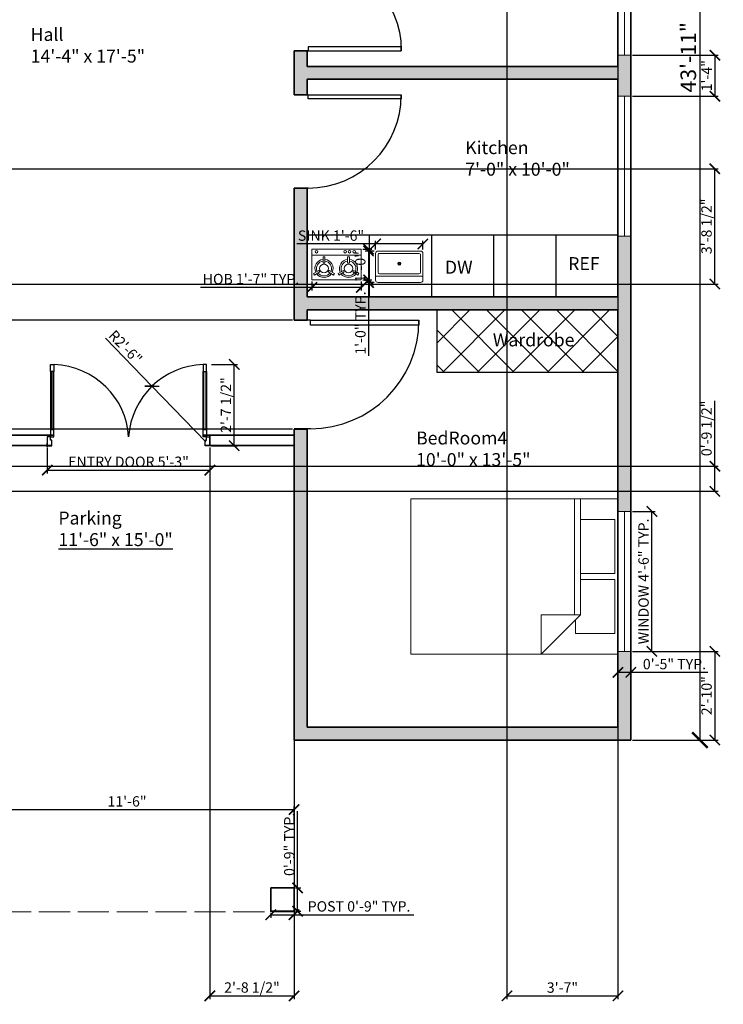
# Model space of a CAD drawing. Units: inches. Extents: x -43 to 8979, y -615 to 8149.
# Tile 2 of 5: x 283 to 555, y -615 to -235. Entities that reach past the tile are written whole.
import ezdxf

# ---------------------------------------------------------------- set-up
doc = ezdxf.new("R2010")
doc.units = ezdxf.units.IN
doc.header["$PDMODE"] = 35
doc.header["$PDSIZE"] = 5
doc.linetypes.add('ACAD_ISO02W100', pattern=[15, 12, -3])
for name, color, linetype, lineweight in [('A-ANNO-DIMS', 2, 'Continuous', 18), ('A-ANNO-TEXT', 7, 'Continuous', 18), ('A-AREA-IDEN', 7, 'Continuous', 25), ('A-COLS', 7, 'Continuous', 35), ('A-DOOR', 4, 'Continuous', 25), ('A-EQPM', 8, 'Continuous', 18), ('A-FLOR-FIXT', 9, 'Continuous', 18), ('A-FLOR-PRKG', 8, 'ACAD_ISO02W100', 18), ('A-FURN', 9, 'Continuous', 18), ('A-GLAZ', 4, 'Continuous', 18), ('A-MILL', 30, 'Continuous', 25), ('A-MILL-PATT', 252, 'Continuous', 13), ('A-WALL', 7, 'Continuous', 35), ('A-WALL-PATT', 1, 'Continuous', 13)]:
    doc.layers.add(name, color=color, linetype=linetype, lineweight=lineweight)
doc.styles.get("Standard").update_dxf_attribs({"font": 'arial.ttf'})
doc.dimstyles.new('ISO-25', dxfattribs={"dimtxt": 4, "dimasz": 4, "dimexe": 1.25, "dimexo": 0.625, "dimtad": 1, "dimlunit": 3, "dimtxsty": 'Standard', "dimblk": 'ARCHTICK', "dimcen": 2.5, "dimadec": 0, "dimazin": 0, "dimtfac": 1, "dimtmove": 0, "dimatfit": 3, "dimfxl": 1, "dimarcsym": 0})

# ---------------------------------------------------------------- blocks, each defined once
blk = doc.blocks.new('*U3')
for p, q in [((0, 0), (0, -6)), ((40, 0), (40, -6))]:
    blk.add_line(p, q)
blk.add_lwpolyline([(0, 0), (0, 40), (1.75, 40), (1.75, 0)], close=True)
blk.add_arc((0, 0), 40, 0, 90)
blk = doc.blocks.new('Bed - Queen')
for p, q in [((0, -80.00003), (0, 0)), ((0, 0), (59.99999, 0)), ((59.99999, 0), (59.99999, -80.00003)), ((7.99999, -1.2), (28.79998, -1.2)), ((7.99999, -14.4), (7.99999, -1.2)), ((28.79998, -1.2), (28.79998, -14.4)), ((31.19999, -1.2), (51.99999, -1.2)), ((31.19999, -14.4), (31.19999, -1.2)), ((51.99999, -1.2), (51.99999, -16.4)), ((0, -14.4), (44.8, -14.4)), ((59.99999, -29.6), (44.8, -14.4)), ((44.8, -14.4), (44.8, -29.6)), ((44.8, -16.8), (0, -16.8)), ((51.99999, -16.4), (46.79936, -16.4)), ((44.8, -29.6), (59.99999, -29.6)), ((59.99999, -80.00003), (0, -80.00003))]:
    blk.add_line(p, q)
blk = doc.blocks.new('Sink-single - 30 in top')
blk.add_line((-15, -3.999996), (15, -3.999996))
for points in [[(-13.5, 0), (13.5, 0)], [(-15, -18.499996), (-15, -1.5)], [(-12.5, -5.499996), (12.5, -5.499996)], [(15, -1.5), (15, -18.499996)], [(-13.5, -17.499996), (-13.5, -6.499996)], [(13.5, -6.499996), (13.5, -17.499996)], [(12.5, -18.499996), (-12.5, -18.499996)], [(13.5, -19.999996), (-13.5, -19.999996)]]:
    blk.add_lwpolyline(points)
for radius in [1, 0.5]:
    blk.add_circle((0, -11.999996), radius)
for centre, radius, start, end in [((-13.5, -1.5), 1.5, 90, 180), ((-12.5, -6.499996), 1, 90, 180), ((12.5, -6.499996), 1, 0, 90), ((13.5, -1.5), 1.5, 0, 90), ((-13.5, -18.499996), 1.5, 180, 270), ((-12.5, -17.499996), 1, 180, 270), ((12.5, -17.499996), 1, 270, 0), ((13.5, -18.499996), 1.5, 270, 0)]:
    blk.add_arc(centre, radius, start, end)
blk = doc.blocks.new('A$C3628088D')
for p, q in [((35, 820), (35, 900)), ((35, 900), (75, 900)), ((75, 900), (75, 820)), ((75, 820), (35, 820)), ((75, 820), (35, 820)), ((35, 820), (35, 180)), ((45, 820), (45, 180)), ((65, 820), (45, 820)), ((65, 180), (65, 820)), ((75, 180), (75, 820)), ((35, 180), (35, 100)), ((75, 180), (35, 180)), ((35, 180), (75, 180)), ((45, 180), (65, 180)), ((75, 100), (75, 180)), ((35, 100), (0, 100)), ((0, 100), (0, 0)), ((35, 60), (35, 100)), ((35, 100), (75, 100)), ((50, 60), (35, 60)), ((50, 50), (50, 60)), ((50, 0), (50, 50)), ((0, 0), (50, 0))]:
    blk.add_line(p, q)
for points in [[(1725, 900), (1725, 820), (1765, 820), (1765, 900)], [(1725, 180), (1725, 820), (1765, 820), (1765, 180)], [(1735, 180), (1735, 820), (1755, 820), (1755, 180)], [(1725, 100), (1725, 180), (1765, 180), (1765, 100)], [(1765, 100), (1800, 100), (1800, 0), (1750, 0), (1750, 50), (1750, 60), (1765, 60)]]:
    blk.add_lwpolyline(points, close=True)
blk.add_arc((1757, 42), 858, 92.1038, 176.1334)
blk.add_ellipse((70, 105), major_axis=(-772, 326), ratio=0.94084, start_param=-2.726592, end_param=-1.199193)
blk = doc.blocks.new('_ArchTick')
at = {"color": 0, "linetype": 'ByBlock', "const_width": 0.15}
blk.add_lwpolyline([(-0.5, -0.5), (0.5, 0.5)], dxfattribs=at)
blk = doc.blocks.new('*D13')
at = {"layer": 'A-ANNO-DIMS', "color": 0, "lineweight": -2, "transparency": 16777216}
for p, q in [((519.68, 14.3), (546.94, 14.3)), ((545.69, 14.3), (545.69, -512.7)), ((519.68, -512.7), (546.94, -512.7))]:
    blk.add_line(p, q, dxfattribs=at)
at = {"layer": 'Defpoints', "color": 0, "transparency": 16777216}
for p in [(519.05, 14.3), (519.05, -512.7), (545.69, -512.7)]:
    blk.add_point(p, dxfattribs=at)
at = {"layer": 'A-ANNO-DIMS', "color": 0, "lineweight": -2, "transparency": 16777216, "xscale": 6, "yscale": 6, "zscale": 6}
for p, rotation in [((545.69, 14.3), 90), ((545.69, -512.7), 270)]:
    blk.add_blockref('_ArchTick', p, dxfattribs=dict(at, rotation=rotation))
at = {"layer": 'A-ANNO-DIMS', "color": 0, "transparency": 16777216, "insert": (541.99, -249.2), "char_height": 6, "attachment_point": 5, "rotation": 90}
blk.add_mtext('43\'-11"', dxfattribs=at)
blk = doc.blocks.new('*D14')
at = {"layer": 'A-ANNO-DIMS', "color": 0, "lineweight": -2, "transparency": 16777216}
for p, q in [((260.05, -539.77), (260.05, -538.32)), ((260.05, -539.57), (389.05, -539.57)), ((389.05, -545.24), (389.05, -538.32))]:
    blk.add_line(p, q, dxfattribs=at)
at = {"layer": 'Defpoints', "color": 0, "transparency": 16777216}
for p in [(389.05, -539.57), (260.05, -540.39), (389.05, -545.87)]:
    blk.add_point(p, dxfattribs=at)
at = {"layer": 'A-ANNO-DIMS', "color": 0, "lineweight": -2, "transparency": 16777216, "xscale": 4, "yscale": 4, "zscale": 4, "rotation": 180}
blk.add_blockref('_ArchTick', (260.05, -539.57), dxfattribs=at)
at = {"layer": 'A-ANNO-DIMS', "color": 0, "lineweight": -2, "transparency": 16777216, "xscale": 4, "yscale": 4, "zscale": 4}
blk.add_blockref('_ArchTick', (389.05, -539.57), dxfattribs=at)
at = {"layer": 'A-ANNO-DIMS', "color": 0, "transparency": 16777216, "insert": (324.55, -536.9), "char_height": 4, "attachment_point": 5}
blk.add_mtext('11\'-6"', dxfattribs=at)
blk = doc.blocks.new('WIN-54x5')
blk.add_line((2.5, 0), (2.5, 54))
blk.add_lwpolyline([(5, 54), (5, 0), (0, 0), (0, 54)], close=True)
blk = doc.blocks.new('COOKTOP-2-BURNER')
for p, q in [((19.04, 11.9), (0, 11.9)), ((0, 0), (0, 11.9)), ((19.04, 0), (19.04, 11.9)), ((0.88, 9.37), (1.24, 9.98)), ((2.94, 8.18), (0.88, 9.37)), ((3.3, 8.8), (1.24, 9.98)), ((2.94, 8.18), (3.3, 8.8)), ((6.55, 8.8), (8.6, 9.98)), ((6.55, 8.8), (6.9, 8.18)), ((6.9, 8.18), (8.96, 9.36)), ((8.6, 9.98), (8.96, 9.36)), ((10.35, 9.37), (10.7, 9.98)), ((12.4, 8.18), (10.35, 9.37)), ((12.76, 8.8), (10.7, 9.98)), ((12.4, 8.18), (12.76, 8.8)), ((16.01, 8.8), (18.06, 9.98)), ((16.01, 8.8), (16.36, 8.18)), ((16.36, 8.18), (18.42, 9.36)), ((18.06, 9.98), (18.42, 9.36)), ((4.56, 5.36), (4.56, 2.99)), ((5.28, 5.36), (4.56, 5.36)), ((5.28, 5.36), (5.28, 2.99)), ((14.02, 5.36), (14.02, 2.99)), ((14.74, 5.36), (14.02, 5.36)), ((14.74, 5.36), (14.74, 2.99)), ((19.04, 2.38), (0, 2.38)), ((19.04, 0), (0, 0)), ((5.28, 2.99), (4.56, 2.99)), ((14.74, 2.99), (14.02, 2.99))]:
    blk.add_line(p, q)
at = {"extrusion": (0, 0, -1)}
for centre, major_axis, start_param, end_param in [((4.92, 7.45), (0, 3.49), 3.2451, 5.134376), ((4.92, 7.45), (-2.04, 2.04), 4.051123, 5.898002), ((4.92, 7.45), (-0.01, 3.49), -0.942584, 0.946692), ((4.92, 7.45), (-2.04, 2.04), 6.145519, 7.992397), ((4.92, 7.45), (-1.2, 1.2), 2.356194490192311, 8.639379797371898), ((4.92, 7.45), (0, 3.49), 1.148752, 3.038029), ((4.92, 7.45), (2.04, 2.04), 0.385932, 2.23281), ((14.38, 7.45), (0, 3.49), 3.244173, 5.13345), ((14.38, 7.45), (2.04, 2.04), 2.480327, 4.327205), ((14.38, 7.45), (0, 3.49), -0.944011, 0.945266), ((14.38, 7.45), (-2.04, 2.04), 6.145519, 7.992397), ((14.38, 7.45), (-1.2, 1.2), 2.356194490192306, 8.639379797371893), ((14.38, 7.45), (0, 3.49), 1.14879, 3.038067), ((14.38, 7.45), (2.04, 2.04), 0.385932, 2.23281), ((2.71, 0.97), (-0.365, 0.365), 2.356194490192189, 8.639379797371776), ((4.5, 0.97), (-0.365, 0.365), 2.356194490192189, 8.639379797371776), ((6.25, 0.97), (-0.365, 0.365), 2.356194490192189, 8.639379797371776), ((17.3, 0.97), (-0.365, 0.365), 2.356194490192189, 8.639379797371776)]:
    blk.add_ellipse(centre, major_axis=major_axis, ratio=1, start_param=start_param, end_param=end_param, dxfattribs=at)
blk = doc.blocks.new('POST-9x9')
blk.add_lwpolyline([(0, 9), (9, 9), (9, 0), (0, 0)], close=True)
blk = doc.blocks.new('*D27')
at = {"layer": 'A-ANNO-DIMS', "color": 0, "lineweight": -2, "transparency": 16777216}
for p, q in [((519.68, -424.48), (528.4, -424.48)), ((527.15, -478.48), (527.15, -424.48)), ((519.68, -478.48), (528.4, -478.48))]:
    blk.add_line(p, q, dxfattribs=at)
at = {"layer": 'Defpoints', "color": 0, "transparency": 16777216}
for p in [(519.05, -424.48), (527.15, -424.48), (519.05, -478.48)]:
    blk.add_point(p, dxfattribs=at)
at = {"layer": 'A-ANNO-DIMS', "color": 0, "lineweight": -2, "transparency": 16777216, "xscale": 4, "yscale": 4, "zscale": 4}
for p, rotation in [((527.15, -424.48), 90), ((527.15, -478.48), 270)]:
    blk.add_blockref('_ArchTick', p, dxfattribs=dict(at, rotation=rotation))
at = {"layer": 'A-ANNO-DIMS', "color": 0, "transparency": 16777216, "insert": (524.46, -451.48), "char_height": 4, "attachment_point": 5, "rotation": 90}
blk.add_mtext('WINDOW 4\'-6" TYP.', dxfattribs=at)
blk = doc.blocks.new('*D28')
at = {"layer": 'A-ANNO-DIMS', "color": 0, "lineweight": -2, "transparency": 16777216}
for p, q in [((514.05, -479.11), (514.05, -487.83)), ((519.05, -479.11), (519.05, -487.83)), ((514.05, -486.58), (519.05, -486.58)), ((519.05, -486.58), (548.69, -486.58))]:
    blk.add_line(p, q, dxfattribs=at)
at = {"layer": 'Defpoints', "color": 0, "transparency": 16777216}
for p in [(514.05, -478.48), (519.05, -478.48), (519.05, -486.58)]:
    blk.add_point(p, dxfattribs=at)
at = {"layer": 'A-ANNO-DIMS', "color": 0, "lineweight": -2, "transparency": 16777216, "xscale": 4, "yscale": 4, "zscale": 4, "rotation": 180}
blk.add_blockref('_ArchTick', (514.05, -486.58), dxfattribs=at)
at = {"layer": 'A-ANNO-DIMS', "color": 0, "lineweight": -2, "transparency": 16777216, "xscale": 4, "yscale": 4, "zscale": 4}
blk.add_blockref('_ArchTick', (519.05, -486.58), dxfattribs=at)
at = {"layer": 'A-ANNO-DIMS', "color": 0, "transparency": 16777216, "insert": (535.87, -483.92), "char_height": 4, "attachment_point": 5}
blk.add_mtext('0\'-5" TYP.', dxfattribs=at)
blk = doc.blocks.new('*D31')
at = {"layer": 'A-ANNO-DIMS', "color": 0, "lineweight": -2, "transparency": 16777216}
for p, q in [((293.74, -399.75), (293.74, -409.79)), ((356.51, -399.75), (356.51, -409.79)), ((293.74, -408.54), (356.51, -408.54))]:
    blk.add_line(p, q, dxfattribs=at)
at = {"layer": 'Defpoints', "color": 0, "transparency": 16777216}
for p in [(293.74, -399.12), (356.51, -399.12), (356.51, -408.54)]:
    blk.add_point(p, dxfattribs=at)
at = {"layer": 'A-ANNO-DIMS', "color": 0, "lineweight": -2, "transparency": 16777216, "xscale": 4, "yscale": 4, "zscale": 4, "rotation": 180}
blk.add_blockref('_ArchTick', (293.74, -408.54), dxfattribs=at)
at = {"layer": 'A-ANNO-DIMS', "color": 0, "lineweight": -2, "transparency": 16777216, "xscale": 4, "yscale": 4, "zscale": 4}
blk.add_blockref('_ArchTick', (356.51, -408.54), dxfattribs=at)
at = {"layer": 'A-ANNO-DIMS', "color": 0, "transparency": 16777216, "insert": (325.13, -405.84), "char_height": 4, "attachment_point": 5}
blk.add_mtext('ENTRY DOOR 5\'-3"', dxfattribs=at)
blk = doc.blocks.new('*D32')
at = {"layer": 'A-ANNO-DIMS', "color": 0, "lineweight": -2, "transparency": 16777216}
for p, q in [((357.14, -367.74), (367.18, -367.74)), ((365.93, -399.12), (365.93, -367.74)), ((357.14, -399.12), (367.18, -399.12))]:
    blk.add_line(p, q, dxfattribs=at)
at = {"layer": 'Defpoints', "color": 0, "transparency": 16777216}
for p in [(356.51, -367.74), (365.93, -367.74), (356.51, -399.12)]:
    blk.add_point(p, dxfattribs=at)
at = {"layer": 'A-ANNO-DIMS', "color": 0, "lineweight": -2, "transparency": 16777216, "xscale": 4, "yscale": 4, "zscale": 4}
for p, rotation in [((365.93, -367.74), 90), ((365.93, -399.12), 270)]:
    blk.add_blockref('_ArchTick', p, dxfattribs=dict(at, rotation=rotation))
at = {"layer": 'A-ANNO-DIMS', "color": 0, "transparency": 16777216, "insert": (363.24, -383.43), "char_height": 4, "attachment_point": 5, "rotation": 90}
blk.add_mtext('2\'-7 1/2"', dxfattribs=at)
blk = doc.blocks.new('*D35')
at = {"layer": 'A-ANNO-DIMS', "color": 0, "lineweight": -2, "transparency": 16777216}
for p, q in [((420.52, -321.23), (390.06, -321.23)), ((420.52, -323.34), (420.52, -319.98)), ((438.75, -321.23), (420.52, -321.23)), ((438.75, -323.34), (438.75, -319.98))]:
    blk.add_line(p, q, dxfattribs=at)
at = {"layer": 'Defpoints', "color": 0, "transparency": 16777216}
for p in [(420.52, -321.23), (420.52, -323.97), (438.75, -323.97)]:
    blk.add_point(p, dxfattribs=at)
at = {"layer": 'A-ANNO-DIMS', "color": 0, "lineweight": -2, "transparency": 16777216, "xscale": 4, "yscale": 4, "zscale": 4, "rotation": 180}
blk.add_blockref('_ArchTick', (420.52, -321.23), dxfattribs=at)
at = {"layer": 'A-ANNO-DIMS', "color": 0, "lineweight": -2, "transparency": 16777216, "xscale": 4, "yscale": 4, "zscale": 4}
blk.add_blockref('_ArchTick', (438.75, -321.23), dxfattribs=at)
at = {"layer": 'A-ANNO-DIMS', "color": 0, "transparency": 16777216, "insert": (403.29, -318.54), "char_height": 4, "attachment_point": 5}
blk.add_mtext('SINK 1\'-6"', dxfattribs=at)
blk = doc.blocks.new('*D36')
at = {"layer": 'A-ANNO-DIMS', "color": 0, "lineweight": -2, "transparency": 16777216}
for p, q in [((419.89, -323.97), (416.53, -323.97)), ((417.78, -323.97), (417.78, -336.12)), ((419.89, -336.12), (416.53, -336.12))]:
    blk.add_line(p, q, dxfattribs=at)
at = {"layer": 'Defpoints', "color": 0, "transparency": 16777216}
for p in [(420.52, -323.97), (417.78, -336.12), (420.52, -336.12)]:
    blk.add_point(p, dxfattribs=at)
at = {"layer": 'A-ANNO-DIMS', "color": 0, "lineweight": -2, "transparency": 16777216, "xscale": 4, "yscale": 4, "zscale": 4}
for p, rotation in [((417.78, -323.97), 90), ((417.78, -336.12), 270)]:
    blk.add_blockref('_ArchTick', p, dxfattribs=dict(at, rotation=rotation))
at = {"layer": 'A-ANNO-DIMS', "color": 0, "transparency": 16777216, "insert": (415.12, -330.04), "char_height": 4, "attachment_point": 5, "rotation": 90}
blk.add_mtext('1\'-0"', dxfattribs=at)
blk = doc.blocks.new('*D37')
at = {"layer": 'A-ANNO-DIMS', "color": 0, "lineweight": -2, "transparency": 16777216}
for p, q in [((395.93, -338.01), (352.85, -338.01)), ((395.93, -335.78), (395.93, -339.26)), ((414.97, -338.01), (395.93, -338.01)), ((414.97, -335.78), (414.97, -339.26))]:
    blk.add_line(p, q, dxfattribs=at)
at = {"layer": 'Defpoints', "color": 0, "transparency": 16777216}
for p in [(395.93, -335.15), (395.93, -338.01), (414.97, -335.15)]:
    blk.add_point(p, dxfattribs=at)
at = {"layer": 'A-ANNO-DIMS', "color": 0, "lineweight": -2, "transparency": 16777216, "xscale": 4, "yscale": 4, "zscale": 4, "rotation": 180}
blk.add_blockref('_ArchTick', (395.93, -338.01), dxfattribs=at)
at = {"layer": 'A-ANNO-DIMS', "color": 0, "lineweight": -2, "transparency": 16777216, "xscale": 4, "yscale": 4, "zscale": 4}
blk.add_blockref('_ArchTick', (414.97, -338.01), dxfattribs=at)
at = {"layer": 'A-ANNO-DIMS', "color": 0, "transparency": 16777216, "insert": (372.39, -335.31), "char_height": 4, "attachment_point": 5}
blk.add_mtext('HOB 1\'-7" TYP.', dxfattribs=at)
blk = doc.blocks.new('*D38')
at = {"layer": 'A-ANNO-DIMS', "color": 0, "lineweight": -2, "transparency": 16777216}
for p, q in [((415.59, -323.25), (419.07, -323.25)), ((417.82, -323.25), (417.82, -335.15)), ((415.59, -335.15), (419.07, -335.15)), ((417.82, -335.15), (417.82, -364.41))]:
    blk.add_line(p, q, dxfattribs=at)
at = {"layer": 'Defpoints', "color": 0, "transparency": 16777216}
for p in [(414.97, -323.25), (414.97, -335.15), (417.82, -335.15)]:
    blk.add_point(p, dxfattribs=at)
at = {"layer": 'A-ANNO-DIMS', "color": 0, "lineweight": -2, "transparency": 16777216, "xscale": 4, "yscale": 4, "zscale": 4}
for p, rotation in [((417.82, -323.25), 90), ((417.82, -335.15), 270)]:
    blk.add_blockref('_ArchTick', p, dxfattribs=dict(at, rotation=rotation))
at = {"layer": 'A-ANNO-DIMS', "color": 0, "transparency": 16777216, "insert": (415.16, -351.78), "char_height": 4, "attachment_point": 5, "rotation": 90}
blk.add_mtext('1\'-0" TYP.', dxfattribs=at)
blk = doc.blocks.new('*D39')
at = {"layer": 'A-ANNO-DIMS', "color": 0, "lineweight": -2, "transparency": 16777216}
for p, q in [((380.02, -579.41), (380.02, -581.38)), ((380.02, -580.13), (389.02, -580.13)), ((389.02, -579.41), (389.02, -581.38)), ((389.02, -580.13), (435.22, -580.13))]:
    blk.add_line(p, q, dxfattribs=at)
at = {"layer": 'Defpoints', "color": 0, "transparency": 16777216}
for p in [(380.02, -578.78), (389.02, -578.78), (389.02, -580.13)]:
    blk.add_point(p, dxfattribs=at)
at = {"layer": 'A-ANNO-DIMS', "color": 0, "lineweight": -2, "transparency": 16777216, "xscale": 4, "yscale": 4, "zscale": 4, "rotation": 180}
blk.add_blockref('_ArchTick', (380.02, -580.13), dxfattribs=at)
at = {"layer": 'A-ANNO-DIMS', "color": 0, "lineweight": -2, "transparency": 16777216, "xscale": 4, "yscale": 4, "zscale": 4}
blk.add_blockref('_ArchTick', (389.02, -580.13), dxfattribs=at)
at = {"layer": 'A-ANNO-DIMS', "color": 0, "transparency": 16777216, "insert": (414.12, -577.44), "char_height": 4, "attachment_point": 5}
blk.add_mtext('POST 0\'-9" TYP.', dxfattribs=at)
blk = doc.blocks.new('*D40')
at = {"layer": 'A-ANNO-DIMS', "color": 0, "lineweight": -2, "transparency": 16777216}
for p, q in [((390.37, -569.78), (390.37, -540.15)), ((389.64, -569.78), (391.62, -569.78)), ((390.37, -578.78), (390.37, -569.78)), ((389.64, -578.78), (391.62, -578.78))]:
    blk.add_line(p, q, dxfattribs=at)
at = {"layer": 'Defpoints', "color": 0, "transparency": 16777216}
for p in [(389.02, -569.78), (390.37, -569.78), (389.02, -578.78)]:
    blk.add_point(p, dxfattribs=at)
at = {"layer": 'A-ANNO-DIMS', "color": 0, "lineweight": -2, "transparency": 16777216, "xscale": 4, "yscale": 4, "zscale": 4}
for p, rotation in [((390.37, -569.78), 90), ((390.37, -578.78), 270)]:
    blk.add_blockref('_ArchTick', p, dxfattribs=dict(at, rotation=rotation))
at = {"layer": 'A-ANNO-DIMS', "color": 0, "transparency": 16777216, "insert": (387.7, -552.97), "char_height": 4, "attachment_point": 5, "rotation": 90}
blk.add_mtext('0\'-9" TYP.', dxfattribs=at)
blk = doc.blocks.new('*D44')
at = {"layer": 'A-ANNO-DIMS', "color": 0, "lineweight": -2, "transparency": 16777216}
for p, q in [((471.21, 4.67), (471.21, -612.69)), ((514.05, 4.67), (514.05, -612.69)), ((471.21, -611.44), (514.05, -611.44))]:
    blk.add_line(p, q, dxfattribs=at)
at = {"layer": 'Defpoints', "color": 0, "transparency": 16777216}
for p in [(471.21, 5.3), (514.05, 5.3), (514.05, -611.44)]:
    blk.add_point(p, dxfattribs=at)
at = {"layer": 'A-ANNO-DIMS', "color": 0, "lineweight": -2, "transparency": 16777216, "xscale": 4, "yscale": 4, "zscale": 4, "rotation": 180}
blk.add_blockref('_ArchTick', (471.21, -611.44), dxfattribs=at)
at = {"layer": 'A-ANNO-DIMS', "color": 0, "lineweight": -2, "transparency": 16777216, "xscale": 4, "yscale": 4, "zscale": 4}
blk.add_blockref('_ArchTick', (514.05, -611.44), dxfattribs=at)
at = {"layer": 'A-ANNO-DIMS', "color": 0, "transparency": 16777216, "insert": (492.63, -608.77), "char_height": 4, "attachment_point": 5}
blk.add_mtext('3\'-7"', dxfattribs=at)
blk = doc.blocks.new('*D46')
at = {"layer": 'A-ANNO-DIMS', "color": 0, "lineweight": -2, "transparency": 16777216}
for p, q in [((7.68, -292.21), (552.7, -292.21)), ((551.45, -336.7), (551.45, -292.21)), ((7.68, -336.7), (552.7, -336.7))]:
    blk.add_line(p, q, dxfattribs=at)
at = {"layer": 'Defpoints', "color": 0, "transparency": 16777216}
for p in [(7.05, -292.21), (551.45, -292.21), (7.05, -336.7)]:
    blk.add_point(p, dxfattribs=at)
at = {"layer": 'A-ANNO-DIMS', "color": 0, "lineweight": -2, "transparency": 16777216, "xscale": 4, "yscale": 4, "zscale": 4}
for p, rotation in [((551.45, -292.21), 90), ((551.45, -336.7), 270)]:
    blk.add_blockref('_ArchTick', p, dxfattribs=dict(at, rotation=rotation))
at = {"layer": 'A-ANNO-DIMS', "color": 0, "transparency": 16777216, "insert": (548.76, -314.45), "char_height": 4, "attachment_point": 5, "rotation": 90}
blk.add_mtext('3\'-8 1/2"', dxfattribs=at)
blk = doc.blocks.new('*D47')
at = {"layer": 'A-ANNO-DIMS', "color": 0, "lineweight": -2, "transparency": 16777216}
for p, q in [((551.45, -407.03), (551.45, -381.83)), ((136.68, -407.03), (552.7, -407.03)), ((551.45, -416.7), (551.45, -407.03)), ((136.68, -416.7), (552.7, -416.7))]:
    blk.add_line(p, q, dxfattribs=at)
at = {"layer": 'Defpoints', "color": 0, "transparency": 16777216}
for p in [(136.05, -407.03), (551.45, -407.03), (136.05, -416.7)]:
    blk.add_point(p, dxfattribs=at)
at = {"layer": 'A-ANNO-DIMS', "color": 0, "lineweight": -2, "transparency": 16777216, "xscale": 4, "yscale": 4, "zscale": 4}
for p, rotation in [((551.45, -407.03), 90), ((551.45, -416.7), 270)]:
    blk.add_blockref('_ArchTick', p, dxfattribs=dict(at, rotation=rotation))
at = {"layer": 'A-ANNO-DIMS', "color": 0, "transparency": 16777216, "insert": (548.76, -392.43), "char_height": 4, "attachment_point": 5, "rotation": 90}
blk.add_mtext('0\'-9 1/2"', dxfattribs=at)
blk = doc.blocks.new('*D50')
at = {"layer": 'A-ANNO-DIMS', "color": 0, "lineweight": -2, "transparency": 16777216}
for p, q in [((519.68, -248.4), (552.7, -248.4)), ((551.45, -248.4), (551.45, -264.22)), ((519.68, -264.22), (552.7, -264.22))]:
    blk.add_line(p, q, dxfattribs=at)
at = {"layer": 'Defpoints', "color": 0, "transparency": 16777216}
for p in [(519.05, -248.4), (519.05, -264.22), (551.45, -264.22)]:
    blk.add_point(p, dxfattribs=at)
at = {"layer": 'A-ANNO-DIMS', "color": 0, "lineweight": -2, "transparency": 16777216, "xscale": 4, "yscale": 4, "zscale": 4}
for p, rotation in [((551.45, -248.4), 90), ((551.45, -264.22), 270)]:
    blk.add_blockref('_ArchTick', p, dxfattribs=dict(at, rotation=rotation))
at = {"layer": 'A-ANNO-DIMS', "color": 0, "transparency": 16777216, "insert": (548.82, -256.31), "char_height": 4, "attachment_point": 5, "rotation": 90}
blk.add_mtext('1\'-4"', dxfattribs=at)
blk = doc.blocks.new('*D51')
at = {"layer": 'A-ANNO-DIMS', "color": 0, "lineweight": -2, "transparency": 16777216}
for p, q in [((519.68, -478.48), (552.7, -478.48)), ((551.45, -478.48), (551.45, -512.7)), ((519.68, -512.7), (552.7, -512.7))]:
    blk.add_line(p, q, dxfattribs=at)
at = {"layer": 'Defpoints', "color": 0, "transparency": 16777216}
for p in [(519.05, -478.48), (519.05, -512.7), (551.45, -512.7)]:
    blk.add_point(p, dxfattribs=at)
at = {"layer": 'A-ANNO-DIMS', "color": 0, "lineweight": -2, "transparency": 16777216, "xscale": 4, "yscale": 4, "zscale": 4}
for p, rotation in [((551.45, -478.48), 90), ((551.45, -512.7), 270)]:
    blk.add_blockref('_ArchTick', p, dxfattribs=dict(at, rotation=rotation))
at = {"layer": 'A-ANNO-DIMS', "color": 0, "transparency": 16777216, "insert": (548.79, -495.59), "char_height": 4, "attachment_point": 5, "rotation": 90}
blk.add_mtext('2\'-10"', dxfattribs=at)
blk = doc.blocks.new('*D52')
at = {"layer": 'A-ANNO-DIMS', "color": 0, "lineweight": -2, "transparency": 16777216}
for p, q in [((356.51, -399.75), (356.51, -612.69)), ((389.05, -399.66), (389.05, -612.69)), ((356.51, -611.44), (389.05, -611.44))]:
    blk.add_line(p, q, dxfattribs=at)
at = {"layer": 'Defpoints', "color": 0, "transparency": 16777216}
for p in [(356.51, -399.12), (389.05, -399.04), (389.05, -611.44)]:
    blk.add_point(p, dxfattribs=at)
at = {"layer": 'A-ANNO-DIMS', "color": 0, "lineweight": -2, "transparency": 16777216, "xscale": 4, "yscale": 4, "zscale": 4, "rotation": 180}
blk.add_blockref('_ArchTick', (356.51, -611.44), dxfattribs=at)
at = {"layer": 'A-ANNO-DIMS', "color": 0, "lineweight": -2, "transparency": 16777216, "xscale": 4, "yscale": 4, "zscale": 4}
blk.add_blockref('_ArchTick', (389.05, -611.44), dxfattribs=at)
at = {"layer": 'A-ANNO-DIMS', "color": 0, "transparency": 16777216, "insert": (372.78, -608.74), "char_height": 4, "attachment_point": 5}
blk.add_mtext('2\'-8 1/2"', dxfattribs=at)
blk = doc.blocks.new('*D56')
at = {"layer": 'A-ANNO-DIMS', "color": 0, "lineweight": -2, "transparency": 16777216}
for p, q in [((388.43, -350.7), (-35.6, -350.7)), ((-34.35, -350.7), (-34.35, -392.7)), ((388.43, -392.7), (-35.6, -392.7))]:
    blk.add_line(p, q, dxfattribs=at)
at = {"layer": 'Defpoints', "color": 0, "transparency": 16777216}
for p in [(389.05, -350.7), (-34.35, -392.7), (389.05, -392.7)]:
    blk.add_point(p, dxfattribs=at)
at = {"layer": 'A-ANNO-DIMS', "color": 0, "lineweight": -2, "transparency": 16777216, "xscale": 4, "yscale": 4, "zscale": 4}
for p, rotation in [((-34.35, -350.7), 90), ((-34.35, -392.7), 270)]:
    blk.add_blockref('_ArchTick', p, dxfattribs=dict(at, rotation=rotation))
at = {"layer": 'A-ANNO-DIMS', "color": 0, "transparency": 16777216, "insert": (-37.01, -371.7), "char_height": 4, "attachment_point": 5, "rotation": 90}
blk.add_mtext('3\'-6"', dxfattribs=at)
blk = doc.blocks.new('*D57')
at = {"layer": 'A-ANNO-DIMS', "color": 0, "lineweight": -2, "transparency": 16777216}
for p in [(316.18, -357.63), (355, -397.66)]:
    blk.add_line(p, (334.15, -376.16), dxfattribs=at)
at = {"layer": 'Defpoints', "color": 0, "transparency": 16777216}
for p in [(334.15, -376.16), (355, -397.66)]:
    blk.add_point(p, dxfattribs=at)
at = {"layer": 'A-ANNO-DIMS', "color": 0, "lineweight": -2, "transparency": 16777216, "xscale": 4, "yscale": 4, "zscale": 4, "rotation": 314.1180906582517}
blk.add_blockref('_ArchTick', (334.15, -376.16), dxfattribs=at)
at = {"layer": 'A-ANNO-DIMS', "color": 0, "transparency": 16777216, "insert": (323.56, -361.41), "char_height": 4, "attachment_point": 5, "rotation": 314.1181}
blk.add_mtext('R2\'-6"', dxfattribs=at)

msp = doc.modelspace()

# ---------------------------------------------------------------- hatches: boundary and pattern name
at = {"layer": 'A-MILL-PATT'}
h = msp.add_hatch(dxfattribs=at)
h.set_pattern_fill('ANSI37', color=256, scale=3)
h.set_pattern_definition([(45, (-529.924, 6e-14), (-6.73519, 6.73519), []), (135, (-529.924, 6e-14), (-6.73519, -6.73519), [])])
h.paths.add_polyline_path([(175.054, -168.703), (7.054, -168.703), (7.054, -192.703), (175.054, -192.703)])
h.paths.add_polyline_path([(175.054, 5.297), (151.054, 5.297), (151.054, -107.703), (175.054, -107.703)])
h.paths.add_polyline_path([(358.054, 5.297), (334.054, 5.297), (334.054, -107.703), (358.054, -107.703)])
h.paths.add_polyline_path([(514.054, -346.703), (444.16, -346.703), (444.16, -370.703), (514.054, -370.703)])
at = {"layer": 'A-WALL-PATT'}
h = msp.add_hatch(color=256, dxfattribs=at)
h.dxf.hatch_style = 1
h.paths.add_polyline_path([(7.054, 5.297), (58.783, 5.297), (58.783, 14.297), (-1.946, 14.297), (-1.946, -51.444), (7.054, -51.444)])
h.paths.add_polyline_path([(7.054, -105.444), (-1.946, -105.444), (-1.946, -238.206), (7.054, -238.206), (7.054, -168.703), (175.054, -168.703), (180.054, -168.703), (186.046, -168.703), (186.046, -163.703), (175.054, -163.703), (7.054, -163.703)])
h.paths.add_polyline_path([(199.054, 14.297), (112.783, 14.297), (112.783, 5.297), (116.889, 5.297), (175.054, 5.297), (175.054, -107.703), (180.054, -107.703), (180.054, -103.21), (180.054, -73.263), (180.054, 5.297), (199.054, 5.297)])
h.paths.add_polyline_path([(276.054, 14.297), (233.054, 14.297), (233.054, 5.297), (252.054, 5.297), (252.054, -102.703), (210.054, -102.703), (210.054, -107.703), (252.054, -107.703), (252.054, -163.703), (222.054, -163.703), (222.054, -168.703), (286.948, -168.703), (286.948, -163.703), (257.054, -163.703), (257.054, -107.703), (299.054, -107.703), (299.054, -102.703), (257.054, -102.703), (257.054, 5.297), (276.054, 5.297)])
h.paths.add_polyline_path([(417.209, 14.297), (310.054, 14.297), (310.054, 5.297), (329.054, 5.297), (329.054, -107.703), (334.054, -107.703), (334.054, 5.297), (417.209, 5.297)])
h.paths.add_polyline_path([(519.054, 14.297), (471.209, 14.297), (471.209, 5.297), (514.054, 5.297), (514.054, -20.367), (519.054, -20.367)])
h.paths.add_polyline_path([(519.054, -74.367), (514.054, -74.367), (514.054, -163.703), (323.054, -163.703), (323.054, -168.703), (329.054, -168.703), (334.054, -168.703), (389.054, -168.703), (389.054, -210.703), (394.054, -210.703), (394.054, -168.703), (514.054, -168.703), (514.054, -194.4), (519.054, -194.4)])
h.paths.add_polyline_path([(519.054, -248.4), (514.054, -248.4), (514.054, -252.703), (394.054, -252.703), (394.054, -246.703), (389.054, -246.703), (389.054, -263.703), (394.054, -263.703), (394.054, -257.703), (514.054, -257.703), (514.054, -264.224), (519.054, -264.224)])
h = msp.add_hatch(color=256, dxfattribs=at)
h.dxf.hatch_style = 1
h.paths.add_polyline_path([(519.054, -318.224), (514.054, -318.224), (514.054, -341.703), (394.054, -341.703), (394.054, -299.703), (389.054, -299.703), (389.054, -341.703), (389.054, -346.703), (389.054, -350.703), (394.054, -350.703), (394.054, -346.703), (514.054, -346.703), (514.054, -424.484), (519.054, -424.484)])
h.paths.add_polyline_path([(519.054, -478.484), (514.054, -478.484), (514.054, -479.58), (514.054, -507.703), (394.054, -507.703), (394.054, -392.703), (389.054, -392.703), (389.054, -512.703), (394.054, -512.703), (519.054, -512.703)])
h.paths.add_polyline_path([(136.054, -421.703), (260.554, -421.703), (260.554, -416.703), (260.554, -345.703), (260.554, -340.703), (249.554, -340.703), (249.554, -345.703), (255.554, -345.703), (255.554, -416.703), (136.054, -416.703), (136.054, -407.032), (127.054, -407.032), (127.054, -512.703), (260.054, -512.703), (260.054, -507.703), (136.054, -507.703)])
h.paths.add_polyline_path([(219.554, -340.703), (180.054, -340.703), (180.054, -234.703), (175.054, -234.703), (175.054, -336.703), (7.054, -336.703), (7.054, -292.206), (-1.946, -292.206), (-1.946, -345.703), (127.054, -345.703), (127.054, -373.032), (136.054, -373.032), (136.054, -345.703), (180.054, -345.703), (219.554, -345.703)])

# ---------------------------------------------------------------- linework, layer by layer
at = {"layer": 'A-DOOR'}
msp.add_line((325.172, -395.037), (325.096, -395.037), dxfattribs=at)
at = {"layer": 'A-FLOR-PRKG'}
for p in [(389.054, -512.703), (260.554, -579.037)]:
    msp.add_line(p, (389.054, -579.037), dxfattribs=at)
at = {"layer": 'A-MILL'}
for p, q in [((394.054, -317.703), (514.054, -317.703)), ((418.054, -317.703), (418.054, -341.703)), ((442.054, -317.703), (442.054, -341.703)), ((466.054, -317.703), (466.054, -341.703)), ((490.054, -317.703), (490.054, -341.703)), ((444.16, -346.703), (444.16, -370.703)), ((444.16, -370.703), (514.054, -370.703))]:
    msp.add_line(p, q, dxfattribs=at)
at = {"layer": 'A-WALL'}
for p, q in [((519.054, 14.297), (519.054, -512.703)), ((514.054, -168.703), (514.054, -252.703)), ((394.054, -246.703), (389.054, -246.703)), ((389.054, -246.703), (389.054, -263.703)), ((394.054, -246.703), (394.054, -252.703)), ((394.054, -252.703), (514.054, -252.703)), ((394.054, -257.703), (514.054, -257.703)), ((394.054, -257.703), (394.054, -263.703)), ((514.054, -257.703), (514.054, -341.703)), ((394.054, -263.703), (389.054, -263.703)), ((394.054, -299.703), (389.054, -299.703)), ((389.054, -299.703), (389.054, -341.703)), ((394.054, -299.703), (394.054, -341.703)), ((389.054, -341.703), (389.054, -346.703)), ((389.054, -341.703), (389.054, -346.703)), ((394.054, -341.703), (514.054, -341.703)), ((389.054, -346.703), (389.054, -350.703)), ((394.054, -346.703), (514.054, -346.703)), ((394.054, -350.703), (394.054, -346.703)), ((514.054, -346.703), (514.054, -507.703)), ((389.054, -350.703), (394.054, -350.703)), ((296.354, -395.037), (260.554, -395.037)), ((389.054, -395.037), (353.897, -395.037)), ((356.46, -399.037), (356.46, -395.037)), ((389.054, -392.703), (394.054, -392.703)), ((389.054, -392.703), (389.054, -512.703)), ((394.054, -392.703), (394.054, -507.703)), ((293.71, -399.554), (293.71, -398.105)), ((295.483, -399.037), (260.554, -399.037)), ((389.054, -399.037), (354.769, -399.037)), ((514.054, -507.703), (394.054, -507.703)), ((394.054, -512.703), (389.054, -512.703)), ((519.054, -512.703), (394.054, -512.703))]:
    msp.add_line(p, q, dxfattribs=at)

# ---------------------------------------------------------------- block references
at = {"layer": 'A-COLS'}
msp.add_blockref('POST-9x9', (380.018, -578.784), dxfattribs=at)
at = {"layer": 'A-DOOR', "rotation": 270}
for p, xscale, yscale, zscale in [((394.45, -246.703), -0.8992725759508509, 0.8992725759508509, 0.8992725759508509), ((394.45, -263.703), 0.8992725759508509, 0.8992725759508509, 0.8992725759508509), ((395.338, -350.703), 1.047254134728217, 1.047254134728217, 1.047254134728217)]:
    msp.add_blockref('*U3', p, dxfattribs=dict(at, xscale=xscale, yscale=yscale, zscale=zscale))
at = {"layer": 'A-DOOR', "xscale": 0.0348744606464488, "yscale": 0.0348744606464488, "zscale": 0.0348744606464488}
msp.add_blockref('A$C3628088D', (293.739, -399.124), dxfattribs=at)
at = {"layer": 'A-EQPM', "rotation": 180}
msp.add_blockref('COOKTOP-2-BURNER', (414.968, -323.254), dxfattribs=at)
at = {"layer": 'A-FLOR-FIXT', "xscale": 0.607825730938939, "yscale": 0.607825730938939, "zscale": 0.607825730938939, "rotation": 180}
msp.add_blockref('Sink-single - 30 in top', (429.637, -336.122), dxfattribs=at)
at = {"layer": 'A-FURN', "rotation": 270}
msp.add_blockref('Bed - Queen', (514.054, -419.58), dxfattribs=at)
at = {"layer": 'A-GLAZ'}
for p in [(514.054, -248.4), (514.054, -318.224), (514.054, -478.484)]:
    msp.add_blockref('WIN-54x5', p, dxfattribs=at)

# ---------------------------------------------------------------- texts
at = {"layer": 'A-ANNO-TEXT', "char_height": 5, "attachment_point": 1}
for s, width, insert in [('REF', 17.27895, (494.848, -326.34)), ('DW', 16.00427, (447.267, -327.724)), ('Wardrobe', 68.19541, (465.776, -355.774))]:
    msp.add_mtext_dynamic_manual_height_columns(s, width=width, gutter_width=12.5, heights=[0], dxfattribs=dict(at, insert=insert))
at = {"layer": 'A-AREA-IDEN', "char_height": 5, "attachment_point": 1}
for s, width, insert in [('Hall\\P14\'-4" x 17\'-5"', 125.28233, (287.365, -237.887)), ('Kitchen\\P7\'-0" x 10\'-0"', 76.04775, (455.111, -281.573)), ('BedRoom4\\P10\'-0" x 13\'-5"', 101.99671, (436.137, -393.64)), ('Parking\\P{\\L11\'-6" x 15\'-0"}', 83.71115, (298.056, -424.528))]:
    msp.add_mtext_dynamic_manual_height_columns(s, width=width, gutter_width=12.5, heights=[0], dxfattribs=dict(at, insert=insert))

# ---------------------------------------------------------------- dimensions: what is measured, and where the dimension line sits
at = {"layer": 'A-ANNO-DIMS'}
for base, p1, p2, angle, override, picture, middle in [((545.685, -512.703), (519.054, 14.297), (519.054, -512.703), 90, {"dimtxt": 6, "dimasz": 6, "dimclrd": 0, "dimclre": 0, "dimclrt": 0}, '*D13', (541.995, -249.203)), ((551.454, -264.224), (519.054, -248.4), (519.054, -264.224), 90, {"dimdec": 1, "dimlfac": 1, "dimrnd": 0, "dimzin": 1, "dimdsep": 46, "dimlunit": 4, "dimfrac": 2}, '*D50', (548.821, -256.312)), ((551.454, -292.206), (7.054, -336.703), (7.054, -292.206), 90, {"dimdec": 1, "dimlfac": 1, "dimrnd": 0, "dimzin": 1, "dimdsep": 46, "dimlunit": 4, "dimfrac": 2}, '*D46', (548.76, -314.454)), ((417.785, -336.122), (420.52, -323.966), (420.52, -336.122), 270, {"dimdec": 1, "dimlfac": 1, "dimrnd": 0, "dimzin": 1, "dimdsep": 46, "dimlunit": 4, "dimfrac": 2}, '*D36', (415.117, -330.044)), ((-34.346, -392.703), (389.054, -350.703), (389.054, -392.703), 90, {"dimdec": 1, "dimlfac": 1, "dimrnd": 0, "dimzin": 1, "dimdsep": 46, "dimlunit": 4, "dimfrac": 2}, '*D56', (-37.014, -371.703)), ((365.929, -367.737), (356.513, -399.124), (356.513, -367.737), 90, {"dimdec": 1, "dimlfac": 1, "dimrnd": 0, "dimzin": 1, "dimdsep": 46, "dimlunit": 4, "dimfrac": 2}, '*D32', (363.236, -383.43)), ((551.454, -407.032), (136.054, -416.703), (136.054, -407.032), 90, {"dimdec": 1, "dimlfac": 1, "dimrnd": 0, "dimzin": 1, "dimdsep": 46, "dimlunit": 4, "dimfrac": 2}, '*D47', (548.761, -392.43)), ((551.454, -512.703), (519.054, -478.484), (519.054, -512.703), 90, {"dimdec": 1, "dimlfac": 1, "dimrnd": 0, "dimzin": 1, "dimdsep": 46, "dimlunit": 4, "dimfrac": 2}, '*D51', (548.787, -495.593))]:
    dim = msp.add_linear_dim(base=base, p1=p1, p2=p2, angle=angle, dimstyle='ISO-25', override=override, dxfattribs=at)
    dim.commit()
    dim.dimension.update_dxf_attribs({"geometry": picture, "text_midpoint": middle})
for base, p1, p2, picture, middle in [((514.054, -611.437), (471.209, 5.297), (514.054, 5.297), '*D44', (492.632, -608.769)), ((389.054, -611.437), (356.513, -399.124), (389.054, -399.037), '*D52', (372.784, -608.744))]:
    dim = msp.add_linear_dim(base=base, p1=p1, p2=p2, dimstyle='ISO-25', override={"dimdec": 1, "dimlfac": 1, "dimrnd": 0, "dimzin": 1, "dimdsep": 46, "dimlunit": 4, "dimfrac": 2}, dxfattribs=at)
    dim.commit()
    dim.dimension.update_dxf_attribs({"geometry": picture, "text_midpoint": middle})
for base, p1, p2, angle, text, picture, middle in [((420.52, -321.231), (438.755, -323.966), (420.52, -323.966), 180, 'SINK <>', '*D35', (403.291, -318.537)), ((417.824, -335.153), (414.968, -323.254), (414.968, -335.153), 270, '<> TYP.', '*D38', (415.157, -351.781)), ((395.93, -338.009), (414.968, -335.153), (395.93, -335.153), 180, 'HOB <> TYP.', '*D37', (372.391, -335.314)), ((527.154, -424.484), (519.054, -478.484), (519.054, -424.484), 90, 'WINDOW <> TYP.', '*D27', (524.46, -451.484)), ((390.369, -569.784), (389.019, -578.784), (389.019, -569.784), 90, '<> TYP.', '*D40', (387.702, -552.968))]:
    dim = msp.add_linear_dim(base=base, p1=p1, p2=p2, angle=angle, text=text, dimstyle='ISO-25', override={"dimdec": 1, "dimlfac": 1, "dimrnd": 0, "dimzin": 1, "dimdsep": 46, "dimlunit": 4, "dimfrac": 2}, dxfattribs=at)
    dim.commit()
    dim.dimension.update_dxf_attribs({"geometry": picture, "text_midpoint": middle})
dim = msp.add_radius_dim(center=(354.996, -397.655), mpoint=(334.155, -376.162), dimstyle='ISO-25', override={"dimdec": 1, "dimlfac": 1, "dimrnd": 0, "dimzin": 1, "dimdsep": 46, "dimlunit": 4, "dimfrac": 2}, dxfattribs=at)
dim.commit()
dim.dimension.update_dxf_attribs({"geometry": '*D57', "text_midpoint": (321.65, -363.266), "dimtype": 164})
for base, p1, p2, text, override, picture, middle in [((356.513, -408.54), (293.739, -399.124), (356.513, -399.124), 'ENTRY DOOR <>', {"dimdec": 1, "dimlfac": 1, "dimrnd": 0, "dimzin": 1, "dimdsep": 46, "dimlunit": 4, "dimfrac": 2}, '*D31', (325.126, -405.844)), ((519.054, -486.584), (514.054, -478.484), (519.054, -478.484), '<> TYP.', {"dimdec": 1, "dimlfac": 1, "dimrnd": 0, "dimzin": 1, "dimdsep": 46, "dimlunit": 4, "dimfrac": 2}, '*D28', (535.87, -483.916)), ((389.054, -539.566), (260.054, -540.391), (389.054, -545.87), '11\'-6"', {"dimclrd": 0, "dimclre": 0, "dimclrt": 0}, '*D14', (324.554, -536.899)), ((389.019, -580.134), (380.019, -578.784), (389.019, -578.784), 'POST <> TYP.', {"dimdec": 1, "dimlfac": 1, "dimrnd": 0, "dimzin": 1, "dimdsep": 46, "dimlunit": 4, "dimfrac": 2}, '*D39', (414.119, -577.44))]:
    dim = msp.add_linear_dim(base=base, p1=p1, p2=p2, text=text, dimstyle='ISO-25', override=override, dxfattribs=at)
    dim.commit()
    dim.dimension.update_dxf_attribs({"geometry": picture, "text_midpoint": middle})

doc.saveas('drawing.dxf')
